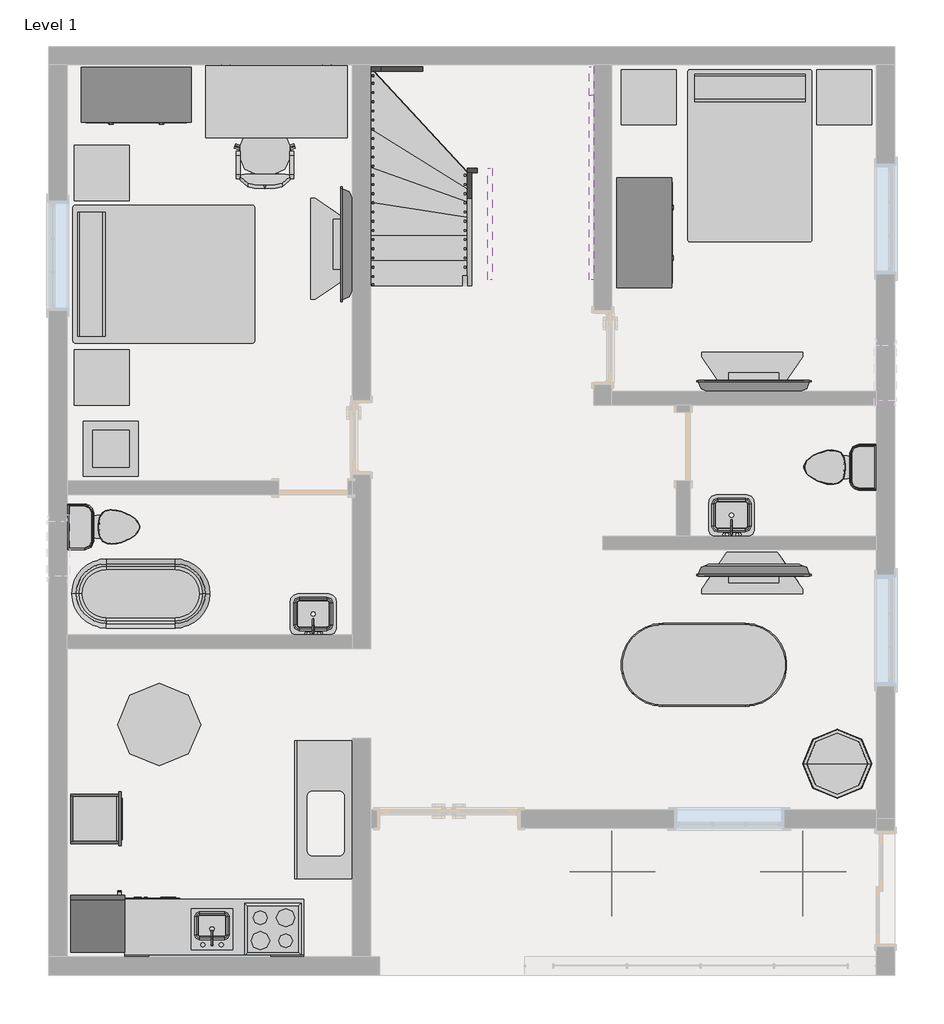
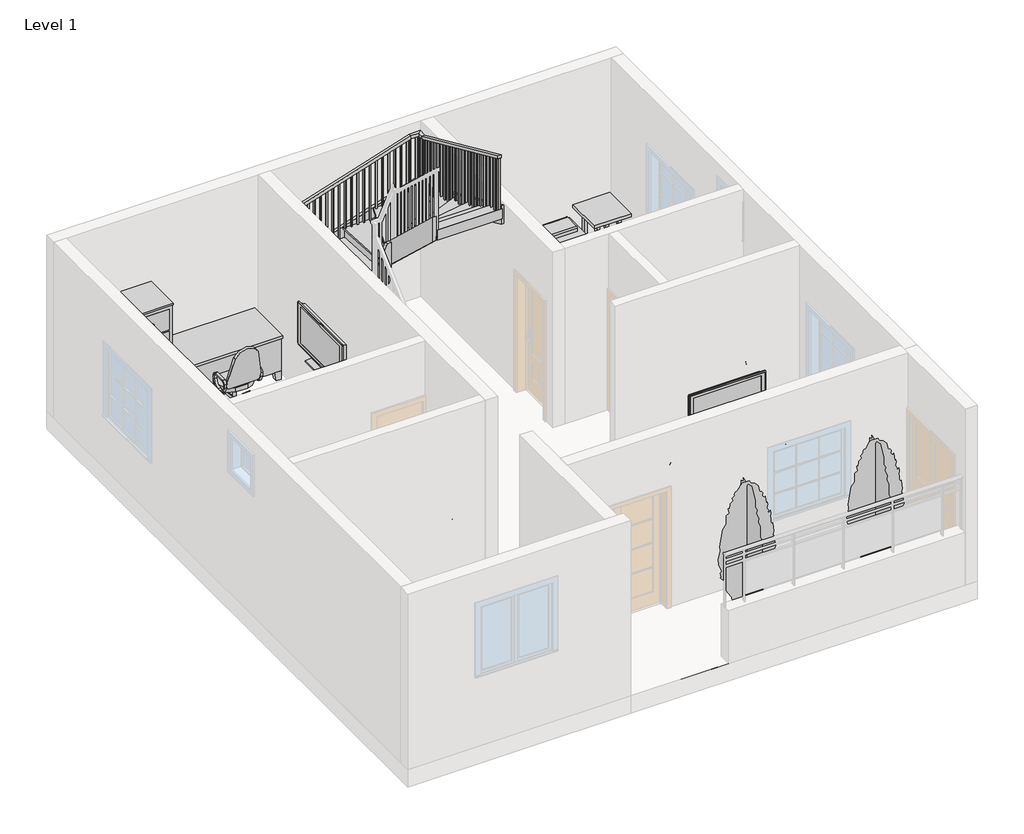
# One storey, part 2 of 2: 22 furniture elements, 8 members, 6 flow terminals, 6 proxies, 2 geographic elements, 1 railing, 1 stair flight.
# Revit data of these elements (continued)
# Element 2 (IfcBuildingElementProxy, "Cook Top-4 Unit2 : 22\" x 20\"") (continued)
#   Materials on its faces: "Steel, Chrome Plated", "Steel, Polished"
# Element 3 (IfcBuildingElementProxy, "Dishwasher : 24\" x 24\" x 34\"")
#   Phase Created = New Construction
#   Materials on its faces: "Steel, Paint Finish, Ivory, Glossy", "Plastic, Opaque Black"
# Element 4 (IfcBuildingElementProxy, "Kitchenette - Medium : Kitchenette - Medium")
#   Phase Created = New Construction
#   Materials on its faces: "Cabinets", "Cabinets - Handles"
# Element 5 (IfcBuildingElementProxy, "Oven Double-Built-in : 21 1/2\" x 39 1/4\" x 21\"")
#   Phase Created = New Construction
#   Materials on its faces: "Steel", "Metal - Stainless Steel, Polished", "Glass"
# Element 6 (IfcBuildingElementProxy, "Refrigerator : 24\" x 25\" LH")
#   Phase Created = New Construction
#   Materials on its faces: "Steel, Paint Finish, Ivory, Glossy", "Steel, Chrome Plated"
# Element 7 (IfcFlowTerminal, "Sink Kitchen-Island : 18\" x 18\"")
#   Mark = "6"
#   Phase Created = New Construction
#   Materials on its faces: "Steel, Polished"
# Element 8 (IfcFlowTerminal, "Sink Vanity-Square : 20\" x 18\"")
#   Mark = "1"
#   Phase Created = New Construction
#   Materials on its faces: "Porcelain, Linen", "Steel, Polished"
# Element 9 (IfcFlowTerminal, "Sink Vanity-Square : 20\" x 18\"")
#   Mark = "2"
#   Phase Created = New Construction
#   Materials on its faces: "Porcelain, Linen", "Steel, Polished"
# Element 10 (IfcFlowTerminal, "Toilet-Domestic-3D : Toilet-Domestic-3D")
#   Mark = "4"
#   Phase Created = New Construction
#   Materials on its faces: "Porcelain, Linen", "Laminate, Linen, Matte"
# Element 11 (IfcFlowTerminal, "Toilet-Domestic-3D : Toilet-Domestic-3D")
#   Mark = "5"
#   Phase Created = New Construction
#   Materials on its faces: "Porcelain, Linen", "Laminate, Linen, Matte"
# Element 12 (IfcFlowTerminal, "Tub-Free Standing-3D : 30\" x 60\"")
#   Mark = "3"
#   Phase Created = New Construction
#   Materials on its faces: "Porcelain, Ivory"
# Element 13 (IfcFurniture, "Bed-Standard.0001 : Double 54\" x 75\"")
#   Phase Created = New Construction
#   Materials on its faces: "Linen, White", "Steel, Chrome Plated"
# Element 14 (IfcFurniture, "Bed-Standard.0001 : Queen 60\" x 79\"")
#   Phase Created = New Construction
#   Materials on its faces: "Linen, White", "Steel, Chrome Plated"
# Element 15 (IfcFurniture, "Chair-Executive : Chair-Executive")
#   Phase Created = New Construction
#   Materials on its faces: "Plastic, Opaque Black", "Textile - Slate Blue"
# Element 16 (IfcFurniture, "Counter Top w Sink Hole : 24\" Depth")
#   Sink Opening Depth = 1' - 2"
#   Sink Location To Wall = 0' - 6"
#   Length = 6' - 6"
#   Sink Location = 3' - 4"
#   Sink Opening Width = 1' - 4"
#   Phase Created = New Construction
#   Materials on its faces: "Counter Top"
# Element 17 (IfcFurniture, "Counter Top w Sink Hole : 24\" Depth")
#   Sink Opening Width = 2' - 3"
#   Sink Opening Depth = 1' - 3"
#   Sink Location To Wall = 0' - 6"
#   Sink Location = 2' - 0"
#   Length = 5' - 0"
#   Phase Created = New Construction
#   Materials on its faces: "Counter Top"
# Element 18 (IfcFurniture, "Desk : 60\" x 30\"")
#   Phase Created = New Construction
#   Materials on its faces: "Steel, Chrome Plated", "Laminate, Ivory, Matte", "Cherry"
# Elements 19, 20 (IfcFurniture, "Dresser : 48\" x 72\" x 24\"")
#   Phase Created = New Construction
#   Materials on its faces: "Laminate, Ivory, Matte", "Cherry", "Laminate - Ivory, Glossy"
# Elements 21, 22, 23 (IfcFurniture, "TV - Flat Screen : 50\"")
#   Stand = yes
#   Phase Created = New Construction
#   Materials on its faces: "TV - Black", "TV - Glass", "TV - Screen"
# Elements 24, 25, 26 (IfcFurniture, "TV Stand : TV Stand")
#   Phase Created = New Construction
#   Materials on its faces: "Melamine - Gray", "Glass - Shelves"
# Element 27 (IfcFurniture, "Table-Coffee : 24\" x 24\" x 24\"")
#   Phase Created = New Construction
#   Materials on its faces: "Glass - Clear, Grey"
# Element 28 (IfcFurniture, "Table-Dining Oval : 36\" x 72\"")
#   Phase Created = New Construction
#   Materials on its faces: "Steel, Chrome Plated", "Glass - Clear, Grey"
# Element 29 (IfcFurniture, "Table-Dining Round w Chairs : 36\" Diameter")
#   Phase Created = New Construction
#   Materials on its faces: "Pine", "Laminate, Linen, Matte"
# Elements 30, 31, 32, 33 (IfcFurniture, "Table-Night Stand : 24\" x 24\" x 30\"")
#   Phase Created = New Construction
#   Materials on its faces: "Birch", "Laminate, Ivory, Matte"
# Element 34 (IfcFurniture, "Table-Round : 36\" Diameter")
#   Phase Created = New Construction
#   Materials on its faces: "Steel, Chrome Plated", "Birch"
# Elements 35, 36 (IfcGeographicElement, "RPC Tree - Conifer : Chinese Juniper - 7'")
#   Phase Created = New Construction
# Elements 37, 38, 39, 40, 41, 42, 43, 44 (IfcMember, "Stringer - 2\" Width")
#   Phase Created = New Construction
# Element 45 (IfcRailing, "Handrail - Rectangular")
#   Phase Created = New Construction
# Element 46 (IfcStairFlight, "2\" Tread 1\" Nosing 1/4\" Riser")
#   Phase Created = New Construction
# Materials
#   "Steel, Chrome Plated": class "Metal", colour RGB 17 17 17, transparency 0, Description = "Chromiuim plated steel", Cost = 0
#   "Steel, Polished": class "Metal", colour RGB 57 57 57, transparency 0, Description = "Polished steel", Cost = 0
#   "Steel, Paint Finish, Ivory, Glossy": class "Metal", colour RGB 247 247 239, transparency 0, Description = "Steel, paint finish, ivory, glossy", Cost = 0
#   "Plastic, Opaque Black": class "Plastic", colour RGB 0 0 0, transparency 0, Description = "Plastic, generic, opaque black", Cost = 0
#   "Cabinets": colour RGB 249 249 249, transparency 0
#   "Cabinets - Handles": class "Metal", colour RGB 57 57 57, transparency 0
#   "Metal - Stainless Steel, Polished": class "Metal", colour RGB 216 216 216, transparency 0
#   "Porcelain, Linen": class "Ceramic", colour RGB 249 239 230, transparency 0, Description = "Porcelain, linen", Cost = 0
#   "Laminate, Linen, Matte": class "Plastic", colour RGB 249 239 230, transparency 0, Description = "Plastic Laminate - Linen, Matte", Cost = 0
#   "Porcelain, Ivory": class "Ceramic", colour RGB 247 247 239, transparency 0, Description = "Porcelain, ivory", Cost = 0
#   "Linen, White": class "Textile", colour RGB 247 247 239, transparency 0, Description = "Linen, white", Cost = 0
#   "Textile - Slate Blue": class "Fabric", colour RGB 98 102 118, transparency 0
#   "Laminate, Ivory, Matte": class "Plastic", colour RGB 247 247 239, transparency 0, Description = "Plastic Laminate - Ivory, Matte", Cost = 0
#   "Cherry": class "Wood", colour RGB 226 177 128, transparency 0, Description = "Prunus Serotina", Cost = 0
#   "Laminate - Ivory, Glossy": colour RGB 247 247 239, transparency 0
#   "Melamine - Gray": class "Wood", colour RGB 49 49 49, transparency 0
#   "Glass - Clear, Grey": class "Glass", colour RGB 252 255 255, transparency 0.64
#   "Pine": class "Wood", colour RGB 223 192 134, transparency 0, Description = "Pinus Echinata", Cost = 0
#   "Birch": class "Wood", colour RGB 224 178 126, transparency 0, Description = "Betula Alleghaniensis", Cost = 0
#   "Steel": class "Metal", colour RGB 247 247 247, transparency 0, Description = "Steel, mill finish", Cost = 0
#   "Glass": class "Glass", colour RGB 0 128 192, transparency 0.75, Description = "Soda Lime Glass", Cost = 0
#   "Counter Top": class "Wood", colour RGB 226 177 128, transparency 0
#   "TV - Black": colour RGB 49 49 49, transparency 0
#   "TV - Glass": colour RGB 157 157 157, transparency 0.9
#   "TV - Screen": colour RGB 0 0 0, transparency 0
#   "Glass - Shelves": class "Glass", colour RGB 167 167 167, transparency 0.9
